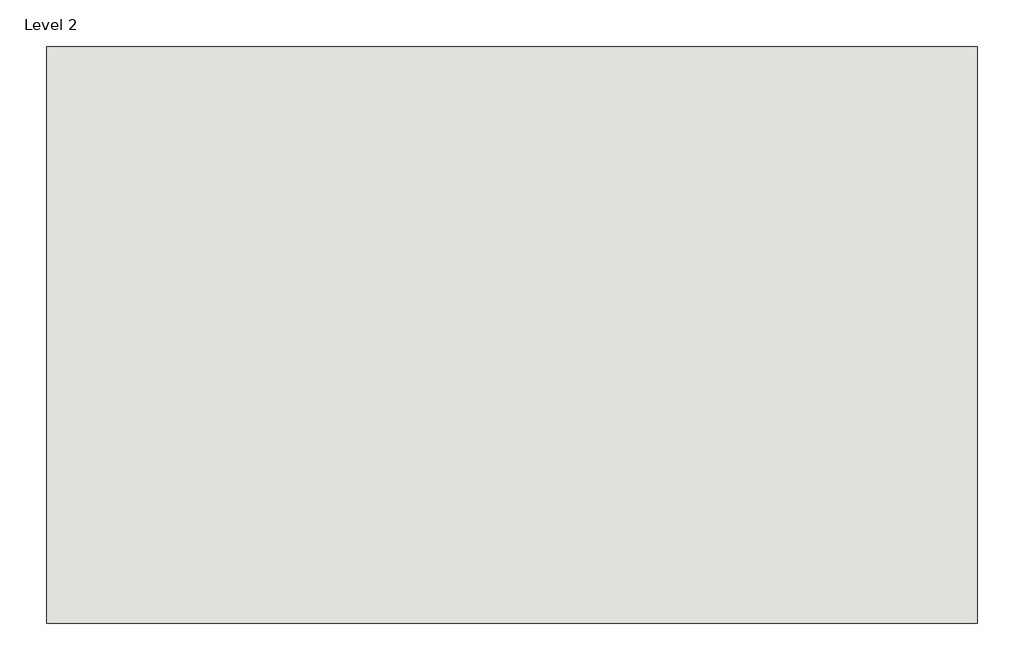
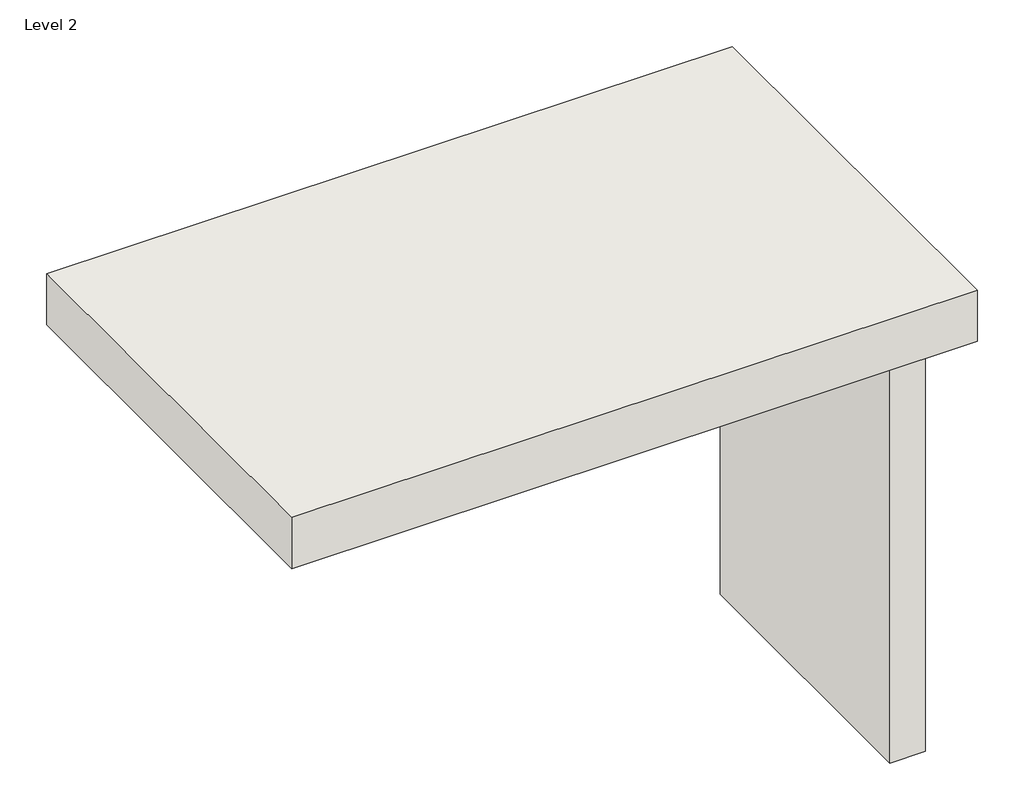
# One storey: 2 walls.
"""IFC4 building model written with IfcOpenShell, lengths in millimetres."""

from ifc_helpers import new_model, si_unit, origin, place, context, project, spatial, faceted_brep, transform, mapped, element, save
from components import walls_7_walls_7_1d2fd38e

model = new_model("IFC4")

# Units and contexts
model_context = context("Model", 3, world=origin())
ifc_project = project(units=[si_unit("LENGTHUNIT", "METRE", prefix="MILLI")], contexts=[model_context])

# Site, building, storey
site = spatial("IfcSite", under=ifc_project)
building = spatial("IfcBuilding", under=site)
storey = spatial("IfcBuildingStorey", under=building, Name="Level 2", Elevation=6096.0)

# Walls
placement = place(None, origin())
element("IfcWall", 1, ObjectType="Generic - 9\"", at=placement, inside=storey, context=model_context, shape_type="Brep", body=[
    faceted_brep([(-9984.4289001, -1538.3180898, 3352.8), (-9984.4289001, -3190.9180898, 3352.8), (-9984.4289001, -3190.9180898, 6096.0), (-9984.4289001, -1739.9180898, 6096.0), (-9984.4289001, -1539.9180898, 6096.0), (-9984.4289001, -1538.3180898, 6096.0), (-9784.4289001, -1538.3180898, 3352.8), (-9784.4289001, -1538.3180898, 6096.0), (-9784.4289001, -3190.9180898, 6096.0), (-9784.4289001, -3190.9180898, 3774.1343037), (-9784.4289001, -3190.9180898, 3352.8)], [[[0, 1, 2, 3, 4, 5]], [[6, 7, 8, 9, 10]], [[1, 0, 6, 10]], [[5, 4, 3, 2, 8, 7]], [[0, 5, 7, 6]], [[1, 10, 9, 8, 2]]]),
])
walls_7_walls_7_shape = walls_7_walls_7_1d2fd38e(model_context)
element("IfcWall", 2, ObjectType="Walls 7 : Walls 7", at=placement, inside=storey, context=model_context, shape_type="MappedRepresentation", body=[
    mapped(walls_7_walls_7_shape, transform((0.0, 0.0, 0.0), x_axis=(1.0, 0.0, 0.0), y_axis=(0.0, 1.0, 0.0), z_axis=(0.0, 0.0, 1.0))),
])

save(model, "model.ifc")

# Revit data of these elements
# Type "Generic - 9\""
#   Layers, outside or top first: 0' - 7.87402" no material (function 1)
# Element 1 (IfcWall, "Generic - 9\"")
#   built-in parameter 1001111 = -9' - 0"
#   Top Offset = 0' - 0"
#   Base Offset = -9' - 0"
#   Unconnected Height = 9' - 0"
#   wall height = 9' - 0"
#   Phase Created = New Construction
#   Base Constraint = Level 2
#   Materials on its faces: "Default Wall"
# Element 2 (IfcWall, "Walls 7 : Walls 7")
#   Phase Created = New Construction
#   Materials on its faces: "Default Wall"
# Materials
#   "Default Wall": colour RGB 80 80 80, transparency 0
